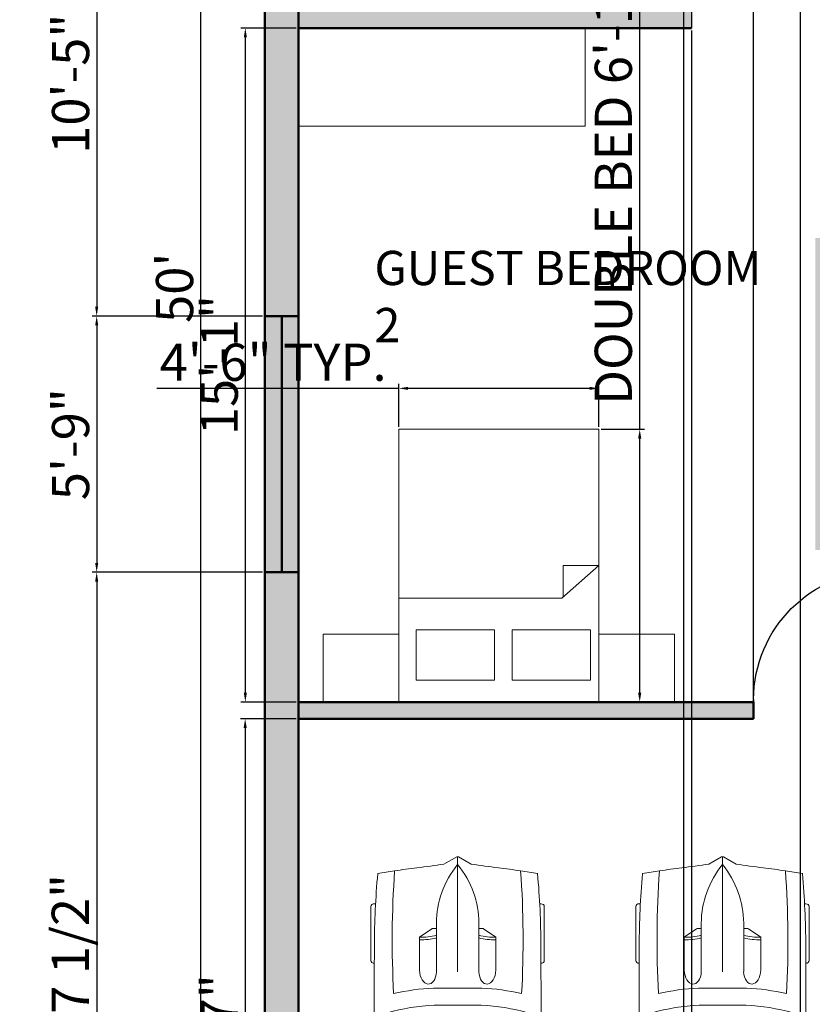
# Model space of a CAD drawing. Units: inches. Extents: x 1344 to 2521, y 3236 to 4924.
# Tile 9 of 14: x 1348 to 1561, y 4260 to 4525. Entities that reach past the tile are written whole.
import ezdxf

# ---------------------------------------------------------------- set-up
doc = ezdxf.new("R2010")
doc.units = ezdxf.units.IN
for name, color, linetype, lineweight in [('A-ANNO-DIMS', 2, 'Continuous', 18), ('A-AREA-IDEN', 3, 'Continuous', 18), ('A-DOOR', 50, 'Continuous', 25), ('A-FURN', 130, 'Continuous', 18), ('A-WALL', 31, 'Continuous', 50), ('A-WALL-PATT', 8, 'Continuous', 13), ('C-PKNG', 193, 'Continuous', 18)]:
    doc.layers.add(name, color=color, linetype=linetype, lineweight=lineweight)
doc.styles.get("Standard").update_dxf_attribs({"font": 'arial.ttf'})
doc.dimstyles.new('ISO-25', dxfattribs={"dimtxt": 10, "dimasz": 2.5, "dimexe": 1.25, "dimexo": 0.625, "dimtad": 1, "dimdec": 0, "dimlunit": 4, "dimtxsty": 'Standard', "dimcen": 2.5, "dimadec": 0, "dimazin": 0, "dimtfac": 1, "dimtdec": 0, "dimtmove": 0, "dimatfit": 3, "dimfxl": 1, "dimarcsym": 0})

# ---------------------------------------------------------------- blocks, each defined once
blk = doc.blocks.new('*U4')
for p, q in [((21.1, 37.41), (21.1, 36.83)), ((46.55, 38.89), (22.35, 38.89)), ((47.8, 37.39), (47.8, 37.41)), ((87.99, 31.87), (74.76, 35.92)), ((134.31, 35.6), (119.29, 31.78)), ((135.45, 37.07), (135.45, 37.41)), ((136.7, 38.89), (160.9, 38.89)), ((162.15, 37.41), (162.15, 36.77)), ((70.03, 31.54), (86.41, 29.35)), ((186.47, -33.5), (186.47, 33.5)), ((188.4, -32.76), (188.4, 32.76)), ((138.42, 29.35), (157.25, 29.35)), ((186.47, 29.35), (167.01, 29.35)), ((164.52, 26.39), (164.52, -26.39)), ((32.27, 11.63), (36.13, 17.17)), ((36.13, 17.17), (50.94, 17.17)), ((29.77, 9.51), (51.68, 9.51)), ((32.12, 9.51), (32.12, 11.15)), ((58.92, -10.77), (58.92, 10.77)), ((66.55, -10.53), (66.55, 10.53)), ((186.47, -10.53), (186.47, 10.53)), ((3.27, 6.13), (0.1, 0.41)), ((82.74, 8.5), (82.74, -8.5)), ((0, 0), (51.68, 0)), ((0.1, -0.41), (3.27, -6.13)), ((29.77, -9.51), (51.68, -9.51)), ((32.12, -9.51), (32.12, -11.15)), ((32.27, -11.63), (36.13, -17.17)), ((36.13, -17.17), (50.94, -17.17)), ((86.41, -29.35), (70.03, -31.54)), ((157.25, -29.35), (138.42, -29.35)), ((167.01, -29.35), (186.47, -29.35)), ((87.99, -31.87), (74.76, -35.92)), ((134.31, -35.6), (119.29, -31.78)), ((21.1, -37.41), (21.1, -36.83)), ((46.55, -38.89), (22.35, -38.89)), ((47.8, -37.39), (47.8, -37.41)), ((135.45, -37.07), (135.45, -37.41)), ((136.7, -38.89), (160.9, -38.89)), ((162.15, -37.41), (162.15, -36.77))]:
    blk.add_line(p, q)
for centre, major_axis, ratio, start_param, end_param in [((266.03, -27.52), (0, 313.31), 0.842304, 1.367076, 1.39176), ((41.19, -490.86), (0, 528.23), 0.842304, 0.00281, 0.075598), ((22.35, 37.41), (0, -1.48), 0.842304, 3.141593, 4.712389), ((64.48, -10555.62), (0, 10593.03), 0.842304, -0.013397, 0.002797), ((46.55, 37.41), (0, 1.48), 0.842304, -1.570796, 0), ((64.48, -10555.62), (0, -10591.55), 0.842304, 3.133765, 3.140441), ((136.7, 37.41), (0, -1.48), 0.842304, 3.141593, 4.712389), ((160.9, 37.41), (0, 1.48), 0.842304, -1.570796, 0), ((180.63, 35.84), (0, 2.22), 0.842304, -0.013017, 1.249894), ((64.48, -10556.36), (0, 10595.31), 0.842304, -0.013397, -0.013017), ((183.98, 33.5), (0, -2.96), 0.842304, 1.570796, 3.128196), ((183.98, 32.76), (0, -5.25), 0.842304, 1.570796, 3.128196), ((135.29, 5.39), (0, 81.77), 0.842304, 1.245306, 1.50788), ((95.79, -3666.35), (0, -3698.24), 0.842304, 3.134049, 3.144098), ((259.18, -27.52), (0, -305.3), 0.842304, 4.528606, 4.561838), ((37.47, -593.96), (0, -623.33), 0.842304, 3.096046, 3.200911), ((134.4, 5.39), (0, -89.78), 0.842304, 4.449482, 4.652344), ((149.6, 2.8), (0, -79.58), 0.842304, 4.372215, 4.640744), ((17.08, 0), (0, 147.02), 0.842304, 4.511394, 4.913384), ((35.91, 0), (0, 147.02), 0.842304, 4.511394, 4.913384), ((167.01, 26.39), (0, 2.96), 0.842304, 0, 1.570796), ((-204.49, 52.4), (0, -250.96), 0.842304, 1.385369, 1.434372), ((13.04, 17.01), (0, 27.42), 0.842304, 4.435146, 4.718221), ((14.2, 17.01), (0, 27.42), 0.842304, 4.435146, 4.718221), ((50.79, 13.34), (6.34, -0.36), 0.603834, -1.395552, 1.581315), ((29.77, -46.66), (0, 56.17), 0.842304, 0, 0.590319), ((32.75, 11.15), (0, 0.74), 0.842304, 0.879714, 1.570796), ((0.62, 0), (0, -0.74), 0.842304, 4.131459, 5.293319), ((29.77, 46.66), (0, 56.17), 0.842304, 2.551274, 3.141593), ((-204.49, -52.4), (0, 250.96), 0.842304, -1.434372, -1.385369), ((149.6, -2.8), (0, -79.58), 0.842304, -1.499151, -1.230623), ((32.75, -11.15), (0, -0.74), 0.842304, 4.712389, 5.403472), ((13.04, -17.01), (0, -27.42), 0.842304, 1.564964, 1.848039), ((14.2, -17.01), (0, -27.42), 0.842304, 1.564964, 1.848039), ((134.4, -5.39), (0, -89.78), 0.842304, -1.510751, -1.307889), ((135.29, -5.39), (0, -81.77), 0.842304, -1.50788, -1.245306), ((259.18, 27.52), (0, 305.3), 0.842304, 1.721348, 1.754579), ((167.01, -26.39), (0, -2.96), 0.842304, 4.712389, 6.283185), ((266.03, 27.52), (0, 313.31), 0.842304, 1.749832, 1.774517), ((37.47, 593.96), (0, -623.33), 0.842304, -0.059319, 0.045547), ((95.79, 3666.35), (0, -3698.24), 0.842304, -0.002505, 0.007544), ((183.98, -33.5), (0, 2.96), 0.842304, 3.15499, 4.712389), ((183.98, -32.76), (0, -5.25), 0.842304, 0.013397, 1.570796), ((41.19, 490.86), (0, -528.23), 0.842304, -0.075598, -0.00281), ((22.35, -37.41), (0, 1.48), 0.842304, 1.570796, 3.141593), ((64.48, 10555.62), (0, 10593.03), 0.842304, 3.138796, 3.15499), ((46.55, -37.41), (0, -1.48), 0.842304, 0, 1.570796), ((64.48, 10555.62), (0, -10591.55), 0.842304, 0.001152, 0.007828), ((136.7, -37.41), (0, -1.48), 0.842304, -1.570796, 0), ((160.9, -37.41), (0, 1.48), 0.842304, 3.141593, 4.712389), ((180.63, -35.84), (0, -2.22), 0.842304, -1.249894, 0.013017), ((64.48, 10556.36), (0, 10595.31), 0.842304, 3.15461, 3.15499)]:
    blk.add_ellipse(centre, major_axis=major_axis, ratio=ratio, start_param=start_param, end_param=end_param)
at = {"extrusion": (0, 0, -1)}
blk.add_ellipse((50.79, -13.34), major_axis=(6.34, 0.36), ratio=0.603834, start_param=-1.395552, end_param=1.581315, dxfattribs=at)
blk = doc.blocks.new('*U2')
for p, q in [((0, 0), (0, -6)), ((40, 0), (40, -6))]:
    blk.add_line(p, q)
blk.add_lwpolyline([(0, 0), (0, 40), (1.75, 40), (1.75, 0)], close=True)
blk.add_arc((0, 0), 40, 0, 90)
blk = doc.blocks.new('*D16')
at = {"layer": 'A-ANNO-DIMS', "color": 0, "lineweight": -2, "transparency": 16777216}
for p, q in [((1412.89, 4753.21), (1394.98, 4753.21)), ((1396.23, 4155.71), (1396.23, 4750.71)), ((1412.89, 4153.21), (1394.98, 4153.21))]:
    blk.add_line(p, q, dxfattribs=at)
at = {"layer": 'A-ANNO-DIMS', "color": 0, "lineweight": 100, "transparency": 16777216}
for points in [[(1395.81, 4750.71), (1396.65, 4750.71), (1396.23, 4753.21)], [(1395.81, 4155.71), (1396.65, 4155.71), (1396.23, 4153.21)]]:
    blk.add_solid(points, dxfattribs=at)
at = {"layer": 'Defpoints', "color": 0, "lineweight": 100, "transparency": 16777216}
for p in [(1396.23, 4753.21), (1413.52, 4753.21), (1413.52, 4153.21)]:
    blk.add_point(p, dxfattribs=at)
at = {"layer": 'A-ANNO-DIMS', "color": 0, "transparency": 16777216, "insert": (1390.5, 4453.21), "char_height": 10, "attachment_point": 5, "rotation": 90}
blk.add_mtext("50'", dxfattribs=at)
blk = doc.blocks.new('*D23')
at = {"layer": 'A-ANNO-DIMS', "color": 0, "lineweight": -2, "transparency": 16777216}
for p, q in [((1421.89, 4523.04), (1406.99, 4523.04)), ((1408.24, 4520.54), (1408.24, 4344.29)), ((1421.89, 4341.79), (1406.99, 4341.79))]:
    blk.add_line(p, q, dxfattribs=at)
at = {"layer": 'A-ANNO-DIMS', "color": 0, "lineweight": 100, "transparency": 16777216}
for points in [[(1407.83, 4520.54), (1408.66, 4520.54), (1408.24, 4523.04)], [(1407.83, 4344.29), (1408.66, 4344.29), (1408.24, 4341.79)]]:
    blk.add_solid(points, dxfattribs=at)
at = {"layer": 'Defpoints', "color": 0, "lineweight": 100, "transparency": 16777216}
for p in [(1422.52, 4523.04), (1408.24, 4341.79), (1422.52, 4341.79)]:
    blk.add_point(p, dxfattribs=at)
at = {"layer": 'A-ANNO-DIMS', "color": 0, "transparency": 16777216, "insert": (1402.51, 4432.42), "char_height": 10, "attachment_point": 5, "rotation": 90}
blk.add_mtext('15\'-1"', dxfattribs=at)
blk = doc.blocks.new('*D24')
at = {"layer": 'A-ANNO-DIMS', "color": 0, "lineweight": -2, "transparency": 16777216}
for p, q in [((1421.89, 4337.29), (1406.95, 4337.29)), ((1408.2, 4334.79), (1408.2, 4164.71)), ((1421.89, 4162.21), (1406.95, 4162.21))]:
    blk.add_line(p, q, dxfattribs=at)
at = {"layer": 'A-ANNO-DIMS', "color": 0, "lineweight": 100, "transparency": 16777216}
for points in [[(1407.78, 4334.79), (1408.61, 4334.79), (1408.2, 4337.29)], [(1407.78, 4164.71), (1408.61, 4164.71), (1408.2, 4162.21)]]:
    blk.add_solid(points, dxfattribs=at)
at = {"layer": 'Defpoints', "color": 0, "lineweight": 100, "transparency": 16777216}
for p in [(1422.52, 4337.29), (1408.2, 4162.21), (1422.52, 4162.21)]:
    blk.add_point(p, dxfattribs=at)
at = {"layer": 'A-ANNO-DIMS', "color": 0, "transparency": 16777216, "insert": (1402.55, 4249.75), "char_height": 10, "attachment_point": 5, "rotation": 90}
blk.add_mtext('14\'-7"', dxfattribs=at)
blk = doc.blocks.new('BED-DOUBLE')
for p, q in [((27.95, 53.78), (27.95, 9.98)), ((27.95, 9.98), (36.68, 0)), ((36.68, 9.56), (28.32, 9.56)), ((36.68, 0), (36.68, 9.56))]:
    blk.add_line(p, q)
for points in [[(0, 0), (73.35, 0), (73.35, 53.78), (0, 53.78)], [(5.91, 28.08), (19.39, 28.08), (19.39, 49.13), (5.91, 49.13)], [(5.91, 2.27), (19.39, 2.27), (19.39, 23.31), (5.91, 23.31)]]:
    blk.add_lwpolyline(points, close=True)
blk = doc.blocks.new('*D63')
at = {"layer": 'A-ANNO-DIMS', "color": 0, "lineweight": -2, "transparency": 16777216}
for p, q in [((1514.3, 4415.14), (1514.3, 4596.59)), ((1503.92, 4415.14), (1515.55, 4415.14)), ((1514.3, 4344.29), (1514.3, 4412.64)), ((1503.92, 4341.79), (1515.55, 4341.79))]:
    blk.add_line(p, q, dxfattribs=at)
at = {"layer": 'A-ANNO-DIMS', "color": 0, "lineweight": 100, "transparency": 16777216}
for points in [[(1513.88, 4412.64), (1514.72, 4412.64), (1514.3, 4415.14)], [(1513.88, 4344.29), (1514.72, 4344.29), (1514.3, 4341.79)]]:
    blk.add_solid(points, dxfattribs=at)
at = {"layer": 'Defpoints', "color": 0, "lineweight": 100, "transparency": 16777216}
for p in [(1503.3, 4415.14), (1514.3, 4415.14), (1503.3, 4341.79)]:
    blk.add_point(p, dxfattribs=at)
at = {"layer": 'A-ANNO-DIMS', "color": 0, "transparency": 16777216, "insert": (1508.5, 4507.12), "char_height": 10, "attachment_point": 5, "rotation": 90}
blk.add_mtext('DOUBLE BED 6\'-1 1/2" TYP.', dxfattribs=at)
blk = doc.blocks.new('*D64')
at = {"layer": 'A-ANNO-DIMS', "color": 0, "lineweight": -2, "transparency": 16777216}
for p, q in [((1449.52, 4415.77), (1449.52, 4427.4)), ((1503.3, 4415.77), (1503.3, 4427.4)), ((1449.52, 4426.15), (1384.41, 4426.15)), ((1500.8, 4426.15), (1452.02, 4426.15))]:
    blk.add_line(p, q, dxfattribs=at)
at = {"layer": 'A-ANNO-DIMS', "color": 0, "lineweight": 100, "transparency": 16777216}
for points in [[(1452.02, 4426.56), (1452.02, 4425.73), (1449.52, 4426.15)], [(1500.8, 4426.56), (1500.8, 4425.73), (1503.3, 4426.15)]]:
    blk.add_solid(points, dxfattribs=at)
at = {"layer": 'Defpoints', "color": 0, "lineweight": 100, "transparency": 16777216}
for p in [(1449.52, 4426.15), (1449.52, 4415.14), (1503.3, 4415.14)]:
    blk.add_point(p, dxfattribs=at)
at = {"layer": 'A-ANNO-DIMS', "color": 0, "transparency": 16777216, "insert": (1415.72, 4431.88), "char_height": 10, "attachment_point": 5}
blk.add_mtext('4\'-6" TYP.', dxfattribs=at)
blk = doc.blocks.new('*D82')
at = {"layer": 'A-ANNO-DIMS', "color": 0, "lineweight": -2, "transparency": 16777216}
for p, q in [((1412.89, 4570.54), (1367.02, 4570.54)), ((1368.27, 4568.04), (1368.27, 4448.1)), ((1412.89, 4445.6), (1367.02, 4445.6))]:
    blk.add_line(p, q, dxfattribs=at)
at = {"layer": 'A-ANNO-DIMS', "color": 0, "lineweight": 100, "transparency": 16777216}
for points in [[(1367.85, 4568.04), (1368.68, 4568.04), (1368.27, 4570.54)], [(1367.85, 4448.1), (1368.68, 4448.1), (1368.27, 4445.6)]]:
    blk.add_solid(points, dxfattribs=at)
at = {"layer": 'Defpoints', "color": 0, "lineweight": 100, "transparency": 16777216}
for p in [(1413.52, 4570.54), (1368.27, 4445.6), (1413.52, 4445.6)]:
    blk.add_point(p, dxfattribs=at)
at = {"layer": 'A-ANNO-DIMS', "color": 0, "transparency": 16777216, "insert": (1362.54, 4508.07), "char_height": 10, "attachment_point": 5, "rotation": 90}
blk.add_mtext('10\'-5"', dxfattribs=at)
blk = doc.blocks.new('*D83')
at = {"layer": 'A-ANNO-DIMS', "color": 0, "lineweight": -2, "transparency": 16777216}
for p, q in [((1412.89, 4445.6), (1367.02, 4445.6)), ((1368.27, 4443.1), (1368.27, 4379.18)), ((1412.89, 4376.68), (1367.02, 4376.68))]:
    blk.add_line(p, q, dxfattribs=at)
at = {"layer": 'A-ANNO-DIMS', "color": 0, "lineweight": 100, "transparency": 16777216}
for points in [[(1367.85, 4443.1), (1368.68, 4443.1), (1368.27, 4445.6)], [(1367.85, 4379.18), (1368.68, 4379.18), (1368.27, 4376.68)]]:
    blk.add_solid(points, dxfattribs=at)
at = {"layer": 'Defpoints', "color": 0, "lineweight": 100, "transparency": 16777216}
for p in [(1413.52, 4445.6), (1368.27, 4376.68), (1413.52, 4376.68)]:
    blk.add_point(p, dxfattribs=at)
at = {"layer": 'A-ANNO-DIMS', "color": 0, "transparency": 16777216, "insert": (1362.54, 4411.14), "char_height": 10, "attachment_point": 5, "rotation": 90}
blk.add_mtext('5\'-9"', dxfattribs=at)
blk = doc.blocks.new('*D84')
at = {"layer": 'A-ANNO-DIMS', "color": 0, "lineweight": -2, "transparency": 16777216}
for p, q in [((1412.89, 4376.68), (1367.02, 4376.68)), ((1368.27, 4374.18), (1368.27, 4155.71)), ((1412.89, 4153.21), (1367.02, 4153.21))]:
    blk.add_line(p, q, dxfattribs=at)
at = {"layer": 'A-ANNO-DIMS', "color": 0, "lineweight": 100, "transparency": 16777216}
for points in [[(1367.85, 4374.18), (1368.68, 4374.18), (1368.27, 4376.68)], [(1367.85, 4155.71), (1368.68, 4155.71), (1368.27, 4153.21)]]:
    blk.add_solid(points, dxfattribs=at)
at = {"layer": 'Defpoints', "color": 0, "lineweight": 100, "transparency": 16777216}
for p in [(1413.52, 4376.68), (1368.27, 4153.21), (1413.52, 4153.21)]:
    blk.add_point(p, dxfattribs=at)
at = {"layer": 'A-ANNO-DIMS', "color": 0, "transparency": 16777216, "insert": (1362.47, 4264.94), "char_height": 10, "attachment_point": 5, "rotation": 90}
blk.add_mtext('18\'-7 1/2"', dxfattribs=at)
blk = doc.blocks.new('*D93')
at = {"layer": 'A-ANNO-DIMS', "color": 0, "lineweight": -2, "transparency": 16777216}
for p, q in [((1526.04, 4667.09), (1526.04, 4106.71)), ((1557.42, 4667.09), (1557.42, 4106.71)), ((1528.54, 4107.96), (1554.92, 4107.96)), ((1557.42, 4107.96), (1611.23, 4107.96))]:
    blk.add_line(p, q, dxfattribs=at)
at = {"layer": 'A-ANNO-DIMS', "color": 0, "lineweight": 100, "transparency": 16777216}
for points in [[(1528.54, 4108.38), (1528.54, 4107.54), (1526.04, 4107.96)], [(1554.92, 4108.38), (1554.92, 4107.54), (1557.42, 4107.96)]]:
    blk.add_solid(points, dxfattribs=at)
at = {"layer": 'Defpoints', "color": 0, "lineweight": 100, "transparency": 16777216}
for p in [(1526.04, 4667.71), (1557.42, 4667.71), (1557.42, 4107.96)]:
    blk.add_point(p, dxfattribs=at)
at = {"layer": 'A-ANNO-DIMS', "color": 0, "transparency": 16777216, "insert": (1585.57, 4113.76), "char_height": 10, "attachment_point": 5}
blk.add_mtext('2\'-7 1/2"', dxfattribs=at)
blk = doc.blocks.new('*D95')
at = {"layer": 'A-ANNO-DIMS', "color": 0, "lineweight": -2, "transparency": 16777216}
for p, q in [((1528.27, 4522.42), (1528.27, 4106.71)), ((1568.27, 4522.42), (1568.27, 4106.71)), ((1530.77, 4107.96), (1565.77, 4107.96))]:
    blk.add_line(p, q, dxfattribs=at)
at = {"layer": 'A-ANNO-DIMS', "color": 0, "lineweight": 100, "transparency": 16777216}
for points in [[(1530.77, 4108.38), (1530.77, 4107.54), (1528.27, 4107.96)], [(1565.77, 4108.38), (1565.77, 4107.54), (1568.27, 4107.96)]]:
    blk.add_solid(points, dxfattribs=at)
at = {"layer": 'Defpoints', "color": 0, "lineweight": 100, "transparency": 16777216}
for p in [(1528.27, 4523.04), (1568.27, 4523.04), (1568.27, 4107.96)]:
    blk.add_point(p, dxfattribs=at)
at = {"layer": 'A-ANNO-DIMS', "color": 0, "transparency": 16777216, "insert": (1548.27, 4113.7), "char_height": 10, "attachment_point": 5}
blk.add_mtext('3\'-4"', dxfattribs=at)
blk = doc.blocks.new('*D99')
at = {"layer": 'A-ANNO-DIMS', "color": 0, "lineweight": -2, "transparency": 16777216}
for p, q in [((1544.94, 4337.92), (1544.94, 4850.71)), ((1547.44, 4849.46), (1577, 4849.46)), ((1579.5, 4337.92), (1579.5, 4850.71)), ((1579.5, 4849.46), (1641.07, 4849.46))]:
    blk.add_line(p, q, dxfattribs=at)
at = {"layer": 'A-ANNO-DIMS', "color": 0, "lineweight": 100, "transparency": 16777216}
for points in [[(1547.44, 4849.88), (1547.44, 4849.04), (1544.94, 4849.46)], [(1577, 4849.88), (1577, 4849.04), (1579.5, 4849.46)]]:
    blk.add_solid(points, dxfattribs=at)
at = {"layer": 'Defpoints', "color": 0, "lineweight": 100, "transparency": 16777216}
for p in [(1579.5, 4849.46), (1544.94, 4337.29), (1579.5, 4337.29)]:
    blk.add_point(p, dxfattribs=at)
at = {"layer": 'A-ANNO-DIMS', "color": 0, "transparency": 16777216, "insert": (1611.53, 4855.26), "char_height": 10, "attachment_point": 5}
blk.add_mtext('2\'-10 1/2"', dxfattribs=at)

msp = doc.modelspace()

# ---------------------------------------------------------------- hatches: boundary and pattern name
at = {"layer": 'A-WALL-PATT'}
h = msp.add_hatch(color=256, dxfattribs=at)
h.dxf.hatch_style = 1
h.paths.add_polyline_path([(1773.52, 4425.27), (1764.52, 4425.27), (1764.52, 4225.22), (1743.16, 4225.22), (1743.16, 4216.22), (1764.52, 4216.22), (1764.52, 4162.21), (1764.52, 4155.88), (1653.6, 4155.88), (1653.6, 4177.58), (1764.52, 4177.58), (1764.52, 4180.4), (1649.25, 4180.4), (1649.25, 4153.21), (1773.52, 4153.21)], flags=17)
h.paths.add_polyline_path([(1598.02, 4180.38), (1593.52, 4180.38), (1589.02, 4180.38), (1589.02, 4162.21), (1565.92, 4162.21), (1565.92, 4153.21), (1598.02, 4153.21)], flags=17)
h.paths.add_polyline_path([(1689.47, 4225.22), (1666.04, 4225.22), (1666.04, 4220.75), (1666.04, 4216.22), (1689.47, 4216.22)], flags=16)
h.paths.add_polyline_path([(1442.43, 4162.21), (1422.52, 4162.21), (1422.52, 4744.21), (1764.52, 4744.21), (1764.52, 4225.22), (1743.16, 4225.22), (1743.16, 4216.22), (1764.52, 4216.22), (1764.52, 4162.21), (1764.52, 4155.88), (1653.6, 4155.88), (1653.6, 4177.58), (1764.52, 4177.58), (1764.52, 4180.4), (1649.25, 4180.4), (1649.25, 4153.21), (1773.52, 4153.21), (1773.52, 4425.27), (1773.52, 4753.21), (1413.52, 4753.21), (1413.52, 4153.21), (1442.43, 4153.21)])
h.paths.add_polyline_path([(1648.69, 4179.48), (1724.08, 4179.48), (1724.08, 4213.98), (1648.69, 4213.98)], flags=25)
h.paths.add_polyline_path([(1609.51, 4245.39), (1659.17, 4245.39), (1659.17, 4264.37), (1609.51, 4264.37)], flags=25)
h.paths.add_polyline_path([(1618.52, 4270.74), (1667.67, 4270.74), (1667.67, 4305.24), (1618.52, 4305.24)], flags=25)
h.paths.add_polyline_path([(1563.46, 4499.55), (1651.73, 4499.55), (1651.73, 4518.53), (1563.46, 4518.53)], flags=25)
h.paths.add_polyline_path([(1439.72, 4433.21), (1521.54, 4433.21), (1521.54, 4467.71), (1439.72, 4467.71)], flags=25)
h.paths.add_polyline_path([(1651.43, 4581.89), (1735.04, 4581.89), (1735.04, 4616.38), (1651.43, 4616.38)], flags=25)
h.paths.add_polyline_path([(1495.42, 4585.56), (1566.53, 4585.56), (1566.53, 4620.06), (1495.42, 4620.06)], flags=25)
h.paths.add_polyline_path([(1677.05, 4699.47), (1729.56, 4699.47), (1729.56, 4718.45), (1677.05, 4718.45)], flags=25)
h.paths.add_polyline_path([(1581.37, 4669.39), (1626.01, 4669.39), (1626.01, 4703.88), (1581.37, 4703.88)], flags=25)
h.paths.add_polyline_path([(1523.21, 4717.23), (1572.85, 4717.23), (1572.85, 4736.21), (1523.21, 4736.21)], flags=25)
h.paths.add_polyline_path([(1432.59, 4685.86), (1482.24, 4685.86), (1482.24, 4704.84), (1432.59, 4704.84)], flags=25)
h = msp.add_hatch(color=256, dxfattribs=at)
h.dxf.hatch_style = 1
h.paths.add_polyline_path([(1528.27, 4527.54), (1422.52, 4527.54), (1422.52, 4523.04), (1499.65, 4523.04), (1528.27, 4523.04)])
h.paths.add_polyline_path([(1575.52, 4626.56), (1571.02, 4626.56), (1571.02, 4527.54), (1568.27, 4527.54), (1568.27, 4523.04), (1575.52, 4523.04)])
h.paths.add_polyline_path([(1413.52, 4445.6), (1422.52, 4445.6), (1422.52, 4570.54), (1413.52, 4570.54)])
h = msp.add_hatch(color=256, dxfattribs=at)
h.dxf.hatch_style = 1
h.paths.add_polyline_path([(1773.52, 4215.79), (1764.52, 4215.79), (1764.52, 4153.21), (1773.52, 4153.21)])
h.paths.add_polyline_path([(1773.52, 4425.27), (1764.52, 4425.27), (1764.52, 4216.22), (1773.52, 4216.22)])
h.paths.add_polyline_path([(1764.52, 4225.22), (1743.16, 4225.22), (1743.16, 4216.22), (1764.52, 4216.22)])
h.paths.add_polyline_path([(1764.52, 4180.4), (1649.25, 4180.4), (1649.25, 4153.21), (1764.52, 4153.21), (1764.52, 4155.88), (1653.6, 4155.88), (1653.6, 4177.58), (1764.52, 4177.58)])
h.paths.add_polyline_path([(1605.63, 4225.22), (1589.02, 4225.22), (1589.02, 4216.22), (1605.63, 4216.22)])
h.paths.add_polyline_path([(1593.52, 4382.64), (1589.02, 4382.64), (1589.02, 4225.22), (1593.52, 4225.22)])
h.paths.add_polyline_path([(1544.94, 4341.79), (1422.52, 4341.79), (1422.52, 4337.29), (1544.94, 4337.29)])
h.paths.add_polyline_path([(1593.52, 4387.14), (1561.57, 4387.14), (1561.57, 4382.64), (1593.52, 4382.64)])
h.paths.add_polyline_path([(1566.07, 4466.57), (1561.57, 4466.57), (1561.57, 4387.14), (1566.07, 4387.14)])

# ---------------------------------------------------------------- linework, layer by layer
at = {"layer": 'A-FURN'}
for points in [[(1499.65, 4523.04), (1422.52, 4523.04), (1422.52, 4496.68), (1499.65, 4496.68)], [(1449.52, 4341.79), (1449.52, 4360.02), (1429.17, 4360.02), (1429.17, 4341.79)], [(1523.64, 4341.79), (1523.64, 4360.02), (1503.3, 4360.02), (1503.3, 4341.79)]]:
    msp.add_lwpolyline(points, close=True, dxfattribs=at)
at = {"layer": 'A-WALL'}
for p, q in [((1528.27, 4523.04), (1422.52, 4523.04)), ((1418.02, 4376.68), (1418.02, 4445.6)), ((1422.52, 4341.79), (1544.94, 4341.79)), ((1422.52, 4337.29), (1544.94, 4337.29))]:
    msp.add_line(p, q, dxfattribs=at)
for points in [[(1565.92, 4153.21), (1773.52, 4153.21), (1773.52, 4753.21), (1413.52, 4753.21), (1413.52, 4153.21), (1442.43, 4153.21)], [(1764.52, 4225.22), (1764.52, 4744.21), (1422.52, 4744.21), (1422.52, 4162.21), (1442.43, 4162.21)]]:
    msp.add_lwpolyline(points, dxfattribs=at)
for points in [[(1413.52, 4376.68), (1422.52, 4376.68), (1422.52, 4445.6), (1413.52, 4445.6)], [(1544.94, 4337.29), (1422.52, 4337.29), (1422.52, 4341.79), (1544.94, 4341.79)]]:
    msp.add_lwpolyline(points, close=True, dxfattribs=at)

# ---------------------------------------------------------------- block references
at = {"layer": 'A-DOOR', "xscale": -1}
msp.add_blockref('*U2', (1568.27, 4529.04), dxfattribs=at)
at = {"layer": 'A-DOOR', "xscale": -0.8638279890898501, "yscale": 0.8638279890898501, "zscale": 0.8638279890898501}
msp.add_blockref('*U2', (1579.5, 4342.47), dxfattribs=at)
at = {"layer": 'A-FURN', "rotation": 90.00000000000055}
msp.add_blockref('BED-DOUBLE', (1503.3, 4341.79), dxfattribs=at)
at = {"layer": 'C-PKNG', "xscale": 0.5992668008637883, "yscale": 0.5992668008637883, "zscale": 0.5992668008637883, "rotation": 270}
for p in [(1465.34, 4300.18), (1536.56, 4300.18)]:
    msp.add_blockref('*U4', p, dxfattribs=at)

# ---------------------------------------------------------------- texts
at = {"layer": 'A-AREA-IDEN', "insert": (1442.96, 4463.13), "char_height": 9.211, "attachment_point": 1}
msp.add_mtext_dynamic_manual_height_columns('GUEST BEDROOM 2', width=108.7809, gutter_width=46.06, heights=[0], dxfattribs=at)

# ---------------------------------------------------------------- dimensions: what is measured, and where the dimension line sits
at = {"layer": 'A-ANNO-DIMS'}
for base, p1, p2, picture, middle in [((1579.5, 4849.46), (1544.94, 4337.29), (1579.5, 4337.29), '*D99', (1611.53, 4855.26)), ((1557.42, 4107.96), (1526.04, 4667.71), (1557.42, 4667.71), '*D93', (1585.57, 4113.76)), ((1568.27, 4107.96), (1528.27, 4523.04), (1568.27, 4523.04), '*D95', (1548.27, 4113.7))]:
    dim = msp.add_linear_dim(base=base, p1=p1, p2=p2, dimstyle='ISO-25', override={"dimdec": 1, "dimlfac": 1, "dimrnd": 0, "dimzin": 1, "dimdsep": 46, "dimlunit": 4, "dimfrac": 2}, dxfattribs=at)
    dim.commit()
    dim.dimension.update_dxf_attribs({"geometry": picture, "text_midpoint": middle})
for base, p1, p2, override, picture, middle in [((1396.23, 4753.21), (1413.52, 4153.21), (1413.52, 4753.21), {"dimclrd": 0, "dimclre": 0, "dimclrt": 0}, '*D16', (1390.5, 4453.21)), ((1368.27, 4445.6), (1413.52, 4570.54), (1413.52, 4445.6), {"dimdec": 1, "dimlfac": 1, "dimrnd": 0, "dimzin": 1, "dimdsep": 46, "dimlunit": 4, "dimfrac": 2}, '*D82', (1362.54, 4508.07)), ((1408.24, 4341.79), (1422.52, 4523.04), (1422.52, 4341.79), {"dimclrd": 0, "dimclre": 0, "dimclrt": 0}, '*D23', (1402.51, 4432.42)), ((1368.27, 4376.68), (1413.52, 4445.6), (1413.52, 4376.68), {"dimdec": 1, "dimlfac": 1, "dimrnd": 0, "dimzin": 1, "dimdsep": 46, "dimlunit": 4, "dimfrac": 2}, '*D83', (1362.54, 4411.14)), ((1368.27, 4153.21), (1413.52, 4376.68), (1413.52, 4153.21), {"dimdec": 1, "dimlfac": 1, "dimrnd": 0, "dimzin": 1, "dimdsep": 46, "dimlunit": 4, "dimfrac": 2}, '*D84', (1362.47, 4264.94)), ((1408.2, 4162.21), (1422.52, 4337.29), (1422.52, 4162.21), {"dimclrd": 0, "dimclre": 0, "dimclrt": 0}, '*D24', (1402.55, 4249.75))]:
    dim = msp.add_linear_dim(base=base, p1=p1, p2=p2, angle=90, dimstyle='ISO-25', override=override, dxfattribs=at)
    dim.commit()
    dim.dimension.update_dxf_attribs({"geometry": picture, "text_midpoint": middle})
for base, p1, p2, angle, text, picture, middle in [((1514.2998, 4415.1429), (1503.2969, 4341.7902), (1503.2969, 4415.1429), 90, 'DOUBLE BED <> TYP.', '*D63', (1508.5009, 4507.1151)), ((1449.52, 4426.15), (1503.3, 4415.14), (1449.52, 4415.14), 180, '<> TYP.', '*D64', (1415.72, 4431.88))]:
    dim = msp.add_linear_dim(base=base, p1=p1, p2=p2, angle=angle, text=text, dimstyle='ISO-25', override={"dimdec": 1, "dimrnd": 0, "dimzin": 1, "dimlunit": 4, "dimfrac": 2}, dxfattribs=at)
    dim.commit()
    dim.dimension.update_dxf_attribs({"geometry": picture, "text_midpoint": middle})

doc.saveas('drawing.dxf')
